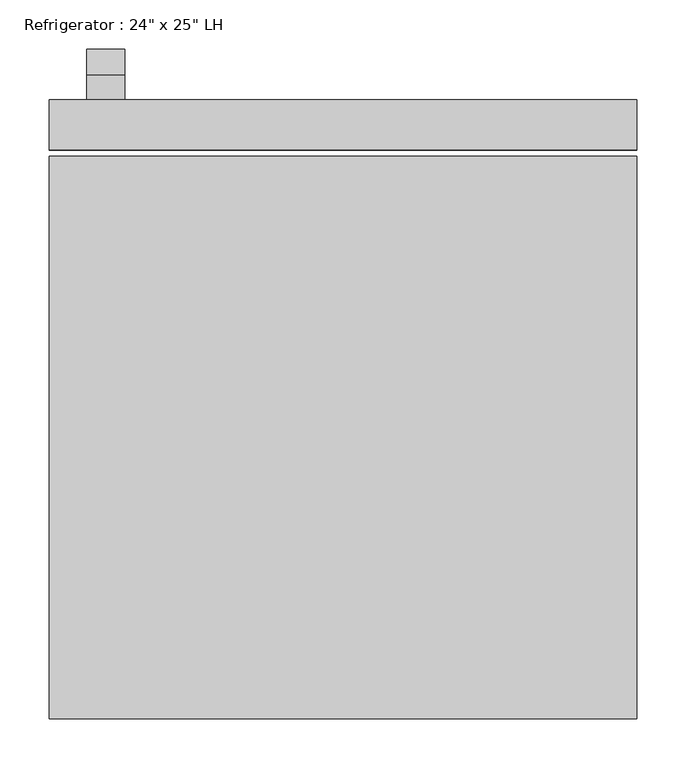
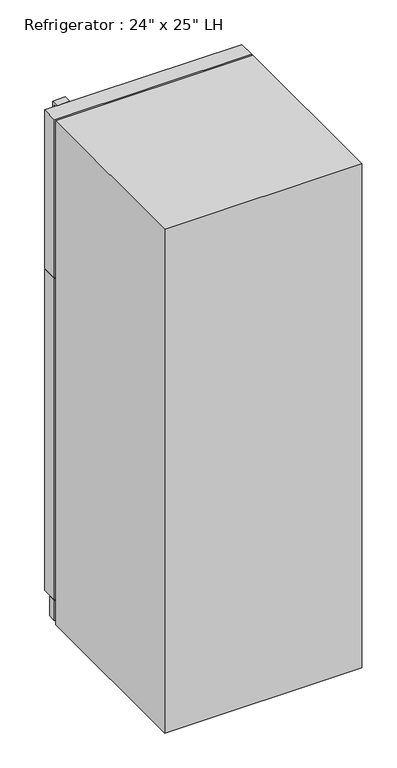
"""IFC4 building model written with IfcOpenShell, lengths in millimetres: proxy geometry."""

from ifc_helpers import new_model, si_unit, frame, origin, origin_with_axes, place, context, project, spatial, polyline, outline, extrude, source, transform, mapped, element, save


def proxy_ec3341c2(model_context):
    return source(origin(), model_context, "Body", "SweptSolid", [
        extrude(outline(polyline([(329.0010285, 1096.9625), (329.0010285, 1103.3125), (379.8010285, 1103.3125), (379.8010285, 900.1125), (351.8949512, 501.0370017), (329.0010285, 501.0370017), (329.0010285, 507.3715334), (345.9723987, 507.3715334), (373.4510285, 900.3342469), (373.4510285, 1096.9625), (329.0010285, 1096.9625)])), frame((-260.35, 0.0, 0.0), z_axis=(1.0, 0.0, 0.0), x_axis=(0.0, 1.0, 0.0)), (0.0, 0.0, 1.0), 38.4332978),
        extrude(outline(polyline([(353.839413, 1612.9), (380.3793675, 1106.4875), (329.7780855, 1106.4875), (329.7780855, 1112.8375), (374.5007207, 1112.8375), (348.6263449, 1606.55), (329.7780855, 1606.55), (329.7780855, 1612.9), (353.839413, 1612.9)])), frame((-260.35, 0.0, 0.0), z_axis=(1.0, 0.0, 0.0), x_axis=(0.0, 1.0, 0.0)), (0.0, 0.0, 1.0), 38.4332978),
        extrude(outline(polyline([(298.45, 278.2010285), (-298.45, 278.2010285), (-298.45, 303.6010285), (298.45, 303.6010285), (298.45, 278.2010285)])), frame((0.0, 0.0, 9.3816357), z_axis=(0.0, 0.0, 1.0), x_axis=(1.0, 0.0, 0.0)), (0.0, 0.0, 1.0), 63.5),
        extrude(outline(polyline([(298.45, 278.2010285), (-298.45, 278.2010285), (-298.45, 329.0010285), (298.45, 329.0010285), (298.45, 278.2010285)])), frame((0.0, 0.0, 76.2), z_axis=(0.0, 0.0, 1.0), x_axis=(1.0, 0.0, 0.0)), (0.0, 0.0, 1.0), 1027.1125),
        extrude(outline(polyline([(298.45, 278.2010285), (-298.45, 278.2010285), (-298.45, 329.0010285), (298.45, 329.0010285), (298.45, 278.2010285)])), frame((0.0, 0.0, 1106.4875), z_axis=(0.0, 0.0, 1.0), x_axis=(1.0, 0.0, 0.0)), (0.0, 0.0, 1.0), 506.4125),
        extrude(outline(polyline([(298.45, -299.6489715), (-298.45, -299.6489715), (-298.45, 271.8510285), (298.45, 271.8510285), (298.45, -299.6489715)])), origin_with_axes(), (0.0, 0.0, 1.0), 1612.9),
    ])


if __name__ == "__main__":
    model = new_model("IFC4")
    model_context = context("Model", 3, world=origin())
    ifc_project = project(units=[si_unit("LENGTHUNIT", "METRE", prefix="MILLI")], contexts=[model_context])
    site = spatial("IfcSite", under=ifc_project)
    building = spatial("IfcBuilding", under=site)
    placement = place(None, origin())
    proxy_shape = proxy_ec3341c2(model_context)
    element("IfcBuildingElementProxy", 1, Name="Refrigerator : 24\" x 25\" LH", ObjectType="Refrigerator : 24\" x 25\" LH", at=placement, inside=building, context=model_context, shape_type="MappedRepresentation", body=[
        mapped(proxy_shape, transform((0.0, 0.0, 0.0), x_axis=(1.0, 0.0, 0.0), y_axis=(0.0, 1.0, 0.0), z_axis=(0.0, 0.0, 1.0))),
    ])
    save(model, "model.ifc")

# Revit data of these elements
# Type "Refrigerator : 24\" x 25\" LH"
#   Label = "REF."
#   Assembly Code = "E1090400"
#   Depth = 2' - 0 3/4"
#   Handle = 0' - 1 1/2"
#   Height = 5' - 3 1/2"
#   Rear Clearance = 0' - 2"
#   Top Door Height = 1' - 8"
#   Width = 1' - 11 1/2"
#   Material = Steel, Paint Finish, Ivory, Glossy
#   Default Elevation = 0
# Element 1 (IfcBuildingElementProxy, "Refrigerator : 24\" x 25\" LH")
#   Materials on its faces: "Steel, Paint Finish, Ivory, Glossy", "Steel, Chrome Plated"
# Materials
#   "Steel, Paint Finish, Ivory, Glossy": class "Metal", colour RGB 247 247 239, transparency 0, Description = "Steel, paint finish, ivory, glossy", Cost = 0
#   "Steel, Chrome Plated": class "Metal", colour RGB 17 17 17, transparency 0, Description = "Chromiuim plated steel", Cost = 0
